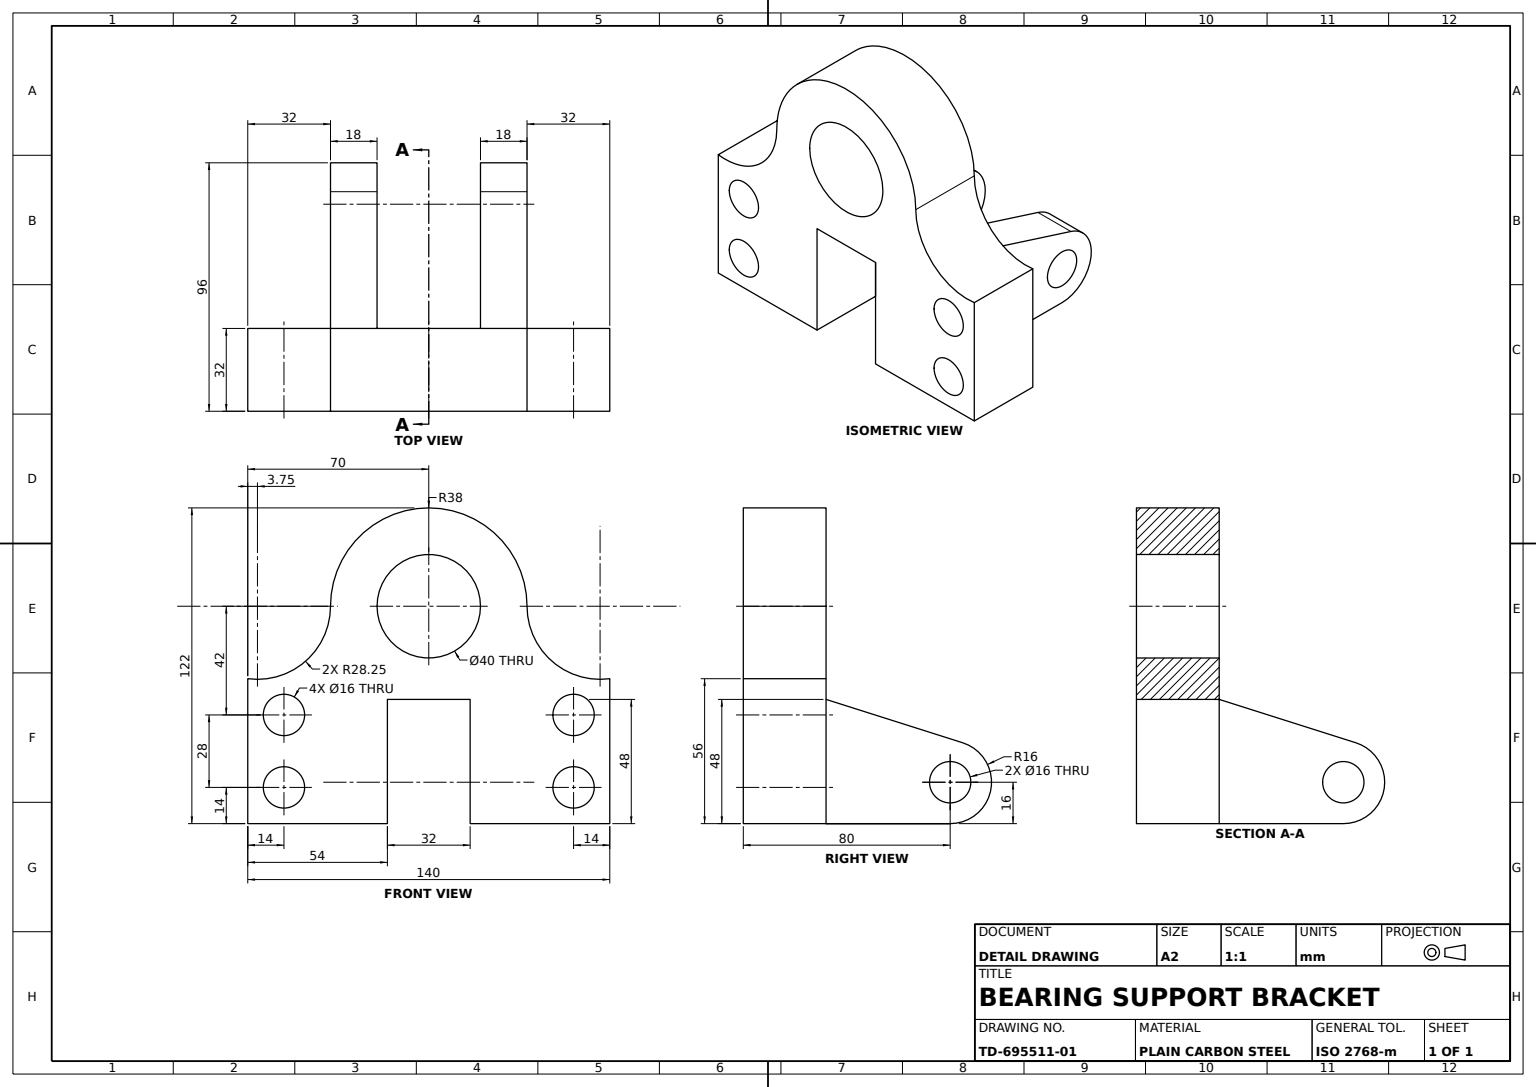
from build123d import *

# Parameters (mm, degrees)
BRACKET_BODY_PROFILE_R   = 20
BRACKET_BODY_PROFILE_R_2 = 8
BRACKET_BODY_32MM_DEPTH  = 16
CLEVIS_LUG_PROFILE_R     = 8
CLEVIS_LUG_18MM_DEPTH    = 18


with BuildPart() as part:
    # Bracket Body Profile → Bracket Body 32mm (new, symmetric)
    with BuildSketch(Plane.XY):
        with BuildLine():
            Line((-16, 0), (16, 0))
            Line((16, 0), (16, -48))
            Line((16, -48), (70, -48))
            Line((70, -48), (70, 8))
            ThreePointArc((70, 8), (47.647244828, 14.739708375), (38, 36))
            ThreePointArc((38, 36), (0, 74), (-38, 36))
            ThreePointArc((-38, 36), (-47.647244828, 14.739708375), (-70, 8))
            Line((-70, 8), (-70, -48))
            Line((-70, -48), (-16, -48))
            Line((-16, -48), (-16, 0))
        make_face()
        with Locations((0, 36)):
            Circle(BRACKET_BODY_PROFILE_R, mode=Mode.SUBTRACT)
        with Locations((56, -34)):
            Circle(BRACKET_BODY_PROFILE_R_2, mode=Mode.SUBTRACT)
        with Locations((56, -6)):
            Circle(BRACKET_BODY_PROFILE_R_2, mode=Mode.SUBTRACT)
        with Locations(Location((-56, -34, 0), (0, 0, 180))):
            Circle(BRACKET_BODY_PROFILE_R_2, mode=Mode.SUBTRACT)
        with Locations(Location((-56, -6, 0), (0, 0, 180))):
            Circle(BRACKET_BODY_PROFILE_R_2, mode=Mode.SUBTRACT)
    extrude(amount=BRACKET_BODY_32MM_DEPTH, both=True)

    # Clevis Lug Profile → Clevis Lug 18mm (add)
    with BuildSketch(Plane(origin=(20, 0, 0), x_dir=(0, 0, -1), z_dir=(1, 0, 0))):
        with BuildLine():
            Line((16, -48), (64, -48))
            ThreePointArc((64, -48), (79.811911333, -34.446111196), (68.834711668, -16.747932498))
            Line((68.834711668, -16.747932498), (16, 0))
            Line((16, 0), (16, -48))
        make_face()
        with Locations((64, -32)):
            Circle(CLEVIS_LUG_PROFILE_R, mode=Mode.SUBTRACT)
    clevis_lug_18mm = extrude(amount=CLEVIS_LUG_18MM_DEPTH)

    # Clevis Lug Mirror: Clevis Lug 18mm across plane
    add(clevis_lug_18mm.mirror(Plane(origin=(0, 0, 0), x_dir=(0, 0, 1), z_dir=(1, 0, 0))))


solid = part.part
